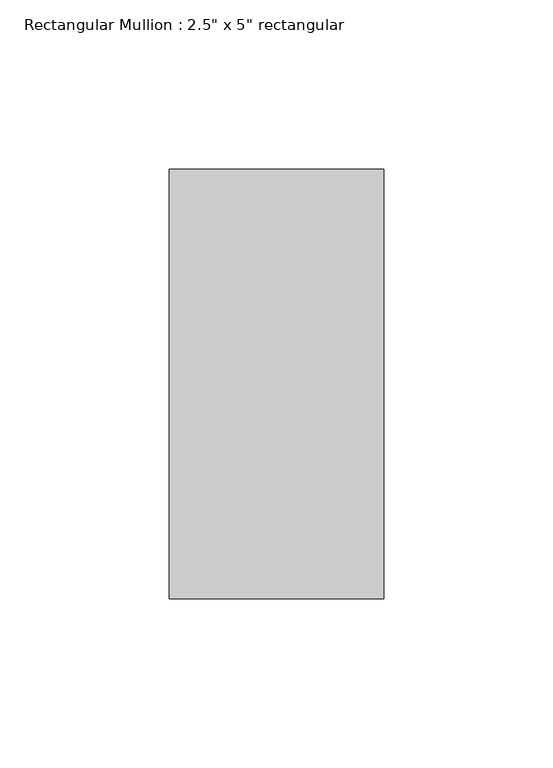
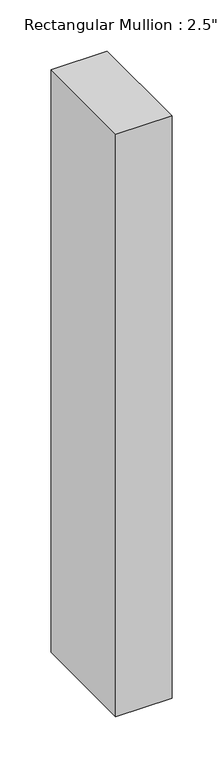
"""IFC4 building model written with IfcOpenShell, lengths in millimetres: member geometry."""

from ifc_helpers import new_model, si_unit, frame, origin, place, context, project, spatial, polyline, outline, extrude, source, transform, mapped, element, save


def member_efb63d8e(model_context):
    return source(origin(), model_context, "Body", "SweptSolid", [
        extrude(outline(polyline([(31.75, 63.5), (31.75, -63.5), (-31.75, -63.5), (-31.75, 63.5), (31.75, 63.5)])), frame((0.0, 0.0, -696.1594531), z_axis=(0.0, 0.0, 1.0), x_axis=(1.0, 0.0, 0.0)), (0.0, 0.0, 1.0), 696.1594531),
    ])


if __name__ == "__main__":
    model = new_model("IFC4")
    model_context = context("Model", 3, world=origin())
    ifc_project = project(units=[si_unit("LENGTHUNIT", "METRE", prefix="MILLI")], contexts=[model_context])
    site = spatial("IfcSite", under=ifc_project)
    building = spatial("IfcBuilding", under=site)
    placement = place(None, origin())
    member_shape = member_efb63d8e(model_context)
    element("IfcMember", 1, ObjectType="Rectangular Mullion : 2.5\" x 5\" rectangular", at=placement, inside=building, context=model_context, shape_type="MappedRepresentation", body=[
        mapped(member_shape, transform((0.0, 0.0, 0.0), x_axis=(1.0, 0.0, 0.0), y_axis=(0.0, 1.0, 0.0), z_axis=(0.0, 0.0, 1.0))),
    ])
    save(model, "model.ifc")

# Revit data of these elements
# Type "Rectangular Mullion : 2.5\" x 5\" rectangular"
#   built-in parameter 1007304 = 0.416667 (stored number, unit not read)
#   built-in parameter 1007301 = 0.104167 (stored number, unit not read)
#   built-in parameter 1007300 = 0.104167 (stored number, unit not read)
# Element 1 (IfcMember, "Rectangular Mullion : 2.5\" x 5\" rectangular")
#   Materials on its faces: "Aluminum"
# Materials
#   "Aluminum": class "Metal", colour RGB 247 247 247, transparency 0, Description = "Aluminum 6061", Cost = 0
